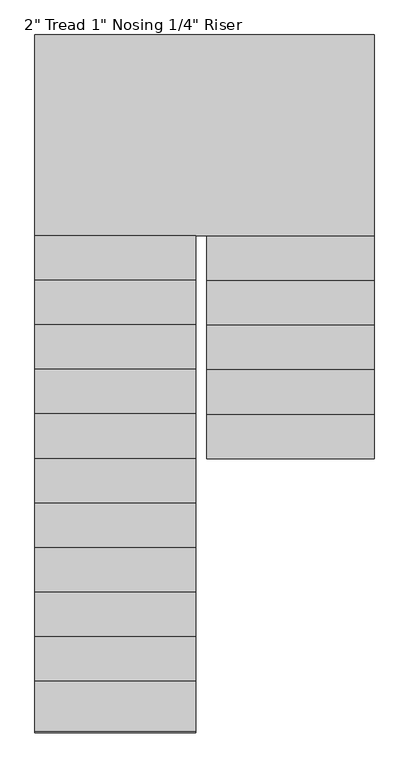
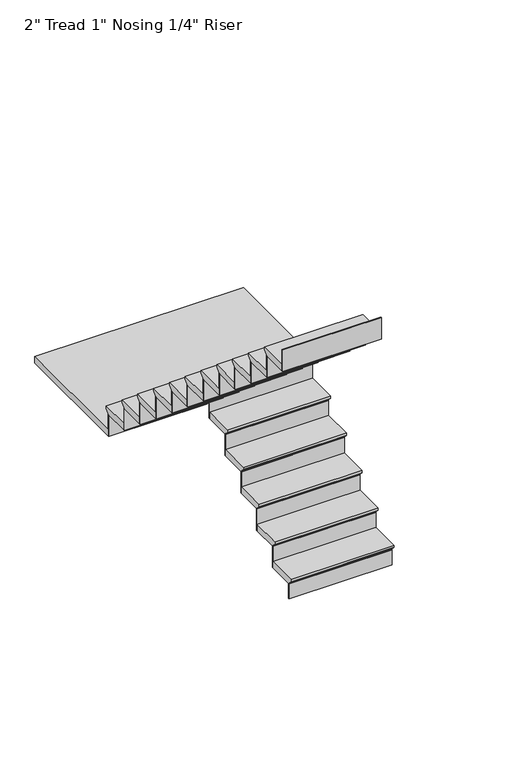
"""IFC4 building model written with IfcOpenShell, lengths in millimetres: stair flight geometry."""

from ifc_helpers import new_model, si_unit, origin, place, context, project, spatial, faceted_brep, source, transform, mapped, element, save


def stair_flight_cacad448(model_context):
    return source(origin(), model_context, "Body", "Brep", [
        faceted_brep([(-3749.597125, 2714.6319226, 27429.8833333), (-3749.597125, 2714.6319226, 27448.9333333), (-4512.2136682, 2714.6319226, 27448.9333333), (-4512.2136682, 2714.6319226, 27429.8833333), (-3749.597125, 2740.0319226, 27404.4833333), (-4512.2136682, 2740.0319226, 27404.4833333), (-3749.597125, 2943.2319226, 27448.9333333), (-4512.2136682, 2943.2319226, 27448.9333333), (-4512.2136682, 2740.0319226, 27398.1333333), (-4512.2136682, 2943.2319226, 27398.1333333), (-3749.597125, 2943.2319226, 27398.1333333), (-3749.597125, 2740.0319226, 27398.1333333)], [[[0, 1, 2, 3]], [[4, 0, 3, 5]], [[2, 1, 6, 7]], [[8, 9, 10, 11]], [[2, 7, 9, 8, 5, 3]], [[8, 11, 4, 5]], [[6, 1, 0, 4, 11, 10]], [[7, 6, 10, 9]]]),
        faceted_brep([(-3749.597125, 2740.0319226, 27398.1333333), (-3749.597125, 2740.0319226, 27279.6), (-3749.597125, 2746.3819226, 27279.6), (-3749.597125, 2746.3819226, 27398.1333333), (-4512.2136682, 2740.0319226, 27398.1333333), (-4512.2136682, 2746.3819226, 27398.1333333), (-4512.2136682, 2746.3819226, 27279.6), (-4512.2136682, 2740.0319226, 27279.6)], [[[0, 1, 2, 3]], [[4, 5, 6, 7]], [[1, 0, 4, 7]], [[2, 1, 7, 6]], [[3, 2, 6, 5]], [[0, 3, 5, 4]]]),
        faceted_brep([(-3749.597125, 2943.2319226, 27567.4666667), (-3749.597125, 2943.2319226, 27398.1333333), (-3749.597125, 2949.5819226, 27398.1333333), (-3749.597125, 2949.5819226, 27567.4666667), (-4512.2136682, 2943.2319226, 27567.4666667), (-4512.2136682, 2949.5819226, 27567.4666667), (-4512.2136682, 2949.5819226, 27398.1333333), (-4512.2136682, 2943.2319226, 27398.1333333)], [[[0, 1, 2, 3]], [[4, 5, 6, 7]], [[1, 0, 4, 7]], [[2, 1, 7, 6]], [[3, 2, 6, 5]], [[0, 3, 5, 4]]]),
        faceted_brep([(-4512.2136682, 2917.8319226, 27618.2666667), (-3749.597125, 2917.8319226, 27618.2666667), (-3749.597125, 3146.4319226, 27618.2666667), (-4512.2136682, 3146.4319226, 27618.2666667), (-4512.2136682, 2943.2319226, 27567.4666667), (-4512.2136682, 3146.4319226, 27567.4666667), (-3749.597125, 3146.4319226, 27567.4666667), (-3749.597125, 2943.2319226, 27567.4666667), (-4512.2136682, 2943.2319226, 27573.8166667), (-4512.2136682, 2917.8319226, 27599.2166667), (-3749.597125, 2943.2319226, 27573.8166667), (-3749.597125, 2917.8319226, 27599.2166667)], [[[0, 1, 2, 3]], [[4, 5, 6, 7]], [[0, 3, 5, 4, 8, 9]], [[4, 7, 10, 8]], [[2, 1, 11, 10, 7, 6]], [[3, 2, 6, 5]], [[11, 1, 0, 9]], [[10, 11, 9, 8]]]),
        faceted_brep([(-3749.597125, 3146.4319226, 27736.8), (-3749.597125, 3146.4319226, 27567.4666667), (-3749.597125, 3152.7819226, 27567.4666667), (-3749.597125, 3152.7819226, 27736.8), (-4512.2136682, 3146.4319226, 27736.8), (-4512.2136682, 3152.7819226, 27736.8), (-4512.2136682, 3152.7819226, 27567.4666667), (-4512.2136682, 3146.4319226, 27567.4666667)], [[[0, 1, 2, 3]], [[4, 5, 6, 7]], [[1, 0, 4, 7]], [[2, 1, 7, 6]], [[3, 2, 6, 5]], [[0, 3, 5, 4]]]),
        faceted_brep([(-4512.2136682, 3121.0319226, 27787.6), (-3749.597125, 3121.0319226, 27787.6), (-3749.597125, 3349.6319226, 27787.6), (-4512.2136682, 3349.6319226, 27787.6), (-4512.2136682, 3146.4319226, 27736.8), (-4512.2136682, 3349.6319226, 27736.8), (-3749.597125, 3349.6319226, 27736.8), (-3749.597125, 3146.4319226, 27736.8), (-4512.2136682, 3146.4319226, 27743.15), (-4512.2136682, 3121.0319226, 27768.55), (-3749.597125, 3146.4319226, 27743.15), (-3749.597125, 3121.0319226, 27768.55)], [[[0, 1, 2, 3]], [[4, 5, 6, 7]], [[0, 3, 5, 4, 8, 9]], [[4, 7, 10, 8]], [[2, 1, 11, 10, 7, 6]], [[3, 2, 6, 5]], [[11, 1, 0, 9]], [[10, 11, 9, 8]]]),
        faceted_brep([(-3749.597125, 3349.6319226, 27906.1333333), (-3749.597125, 3349.6319226, 27736.8), (-3749.597125, 3355.9819226, 27736.8), (-3749.597125, 3355.9819226, 27906.1333333), (-4512.2136682, 3349.6319226, 27906.1333333), (-4512.2136682, 3355.9819226, 27906.1333333), (-4512.2136682, 3355.9819226, 27736.8), (-4512.2136682, 3349.6319226, 27736.8)], [[[0, 1, 2, 3]], [[4, 5, 6, 7]], [[1, 0, 4, 7]], [[2, 1, 7, 6]], [[3, 2, 6, 5]], [[0, 3, 5, 4]]]),
        faceted_brep([(-4512.2136682, 3324.2319226, 27956.9333333), (-3749.597125, 3324.2319226, 27956.9333333), (-3749.597125, 3552.8319226, 27956.9333333), (-4512.2136682, 3552.8319226, 27956.9333333), (-4512.2136682, 3349.6319226, 27906.1333333), (-4512.2136682, 3552.8319226, 27906.1333333), (-3749.597125, 3552.8319226, 27906.1333333), (-3749.597125, 3349.6319226, 27906.1333333), (-4512.2136682, 3349.6319226, 27912.4833333), (-4512.2136682, 3324.2319226, 27937.8833333), (-3749.597125, 3349.6319226, 27912.4833333), (-3749.597125, 3324.2319226, 27937.8833333)], [[[0, 1, 2, 3]], [[4, 5, 6, 7]], [[0, 3, 5, 4, 8, 9]], [[4, 7, 10, 8]], [[2, 1, 11, 10, 7, 6]], [[3, 2, 6, 5]], [[11, 1, 0, 9]], [[10, 11, 9, 8]]]),
        faceted_brep([(-3749.597125, 3552.8319226, 28075.4666667), (-3749.597125, 3552.8319226, 27906.1333333), (-3749.597125, 3559.1819226, 27906.1333333), (-3749.597125, 3559.1819226, 28075.4666667), (-4512.2136682, 3552.8319226, 28075.4666667), (-4512.2136682, 3559.1819226, 28075.4666667), (-4512.2136682, 3559.1819226, 27906.1333333), (-4512.2136682, 3552.8319226, 27906.1333333)], [[[0, 1, 2, 3]], [[4, 5, 6, 7]], [[1, 0, 4, 7]], [[2, 1, 7, 6]], [[3, 2, 6, 5]], [[0, 3, 5, 4]]]),
        faceted_brep([(-4512.2136682, 3527.4319226, 28126.2666667), (-3749.597125, 3527.4319226, 28126.2666667), (-3749.597125, 3756.0319226, 28126.2666667), (-4512.2136682, 3756.0319226, 28126.2666667), (-4512.2136682, 3552.8319226, 28075.4666667), (-4512.2136682, 3756.0319226, 28075.4666667), (-3749.597125, 3756.0319226, 28075.4666667), (-3749.597125, 3552.8319226, 28075.4666667), (-4512.2136682, 3552.8319226, 28081.8166667), (-4512.2136682, 3527.4319226, 28107.2166667), (-3749.597125, 3552.8319226, 28081.8166667), (-3749.597125, 3527.4319226, 28107.2166667)], [[[0, 1, 2, 3]], [[4, 5, 6, 7]], [[0, 3, 5, 4, 8, 9]], [[4, 7, 10, 8]], [[2, 1, 11, 10, 7, 6]], [[3, 2, 6, 5]], [[11, 1, 0, 9]], [[10, 11, 9, 8]]]),
        faceted_brep([(-3749.597125, 3756.0319226, 28244.8), (-3749.597125, 3756.0319226, 28075.4666667), (-3749.597125, 3762.3819226, 28075.4666667), (-3749.597125, 3762.3819226, 28244.8), (-4512.2136682, 3756.0319226, 28244.8), (-4512.2136682, 3762.3819226, 28244.8), (-4512.2136682, 3762.3819226, 28075.4666667), (-4512.2136682, 3756.0319226, 28075.4666667)], [[[0, 1, 2, 3]], [[4, 5, 6, 7]], [[1, 0, 4, 7]], [[2, 1, 7, 6]], [[3, 2, 6, 5]], [[0, 3, 5, 4]]]),
        faceted_brep([(-4563.0136682, 3705.2319226, 28295.6), (-4563.0136682, 3730.6319226, 28295.6), (-3749.597125, 3730.6319226, 28295.6), (-3749.597125, 4645.0319226, 28295.6), (-5295.0246464, 4645.0319226, 28295.6), (-5295.0246464, 3705.2319226, 28295.6), (-4563.0136682, 3730.6319226, 28244.8), (-4563.0136682, 3705.2319226, 28244.8), (-5295.0246464, 3705.2319226, 28244.8), (-5295.0246464, 4645.0319226, 28244.8), (-3749.597125, 4645.0319226, 28244.8), (-3749.597125, 3756.0319226, 28244.8), (-4512.2136682, 3756.0319226, 28244.8), (-4512.2136682, 3730.6319226, 28244.8), (-4512.2136682, 3730.6319226, 28276.55), (-3749.597125, 3730.6319226, 28276.55), (-4512.2136682, 3756.0319226, 28251.15), (-3749.597125, 3756.0319226, 28251.15)], [[[0, 1, 2, 3, 4, 5]], [[6, 7, 8, 9, 10, 11, 12, 13]], [[1, 0, 7, 6]], [[2, 1, 6, 13, 14, 15]], [[13, 12, 16, 14]], [[12, 11, 17, 16]], [[3, 2, 15, 17, 11, 10]], [[4, 3, 10, 9]], [[5, 4, 9, 8]], [[0, 5, 8, 7]], [[17, 15, 14, 16]]]),
        faceted_brep([(-5295.0246464, 3705.2319226, 28414.1333333), (-5295.0246464, 3705.2319226, 28244.8), (-5295.0246464, 3698.8819226, 28244.8), (-5295.0246464, 3698.8819226, 28414.1333333), (-4563.0136682, 3705.2319226, 28414.1333333), (-4563.0136682, 3698.8819226, 28414.1333333), (-4563.0136682, 3698.8819226, 28244.8), (-4563.0136682, 3705.2319226, 28244.8)], [[[0, 1, 2, 3]], [[4, 5, 6, 7]], [[1, 0, 4, 7]], [[2, 1, 7, 6]], [[3, 2, 6, 5]], [[0, 3, 5, 4]]]),
        faceted_brep([(-4563.0136682, 3730.6319226, 28464.9333333), (-5295.0246464, 3730.6319226, 28464.9333333), (-5295.0246464, 3502.0319226, 28464.9333333), (-4563.0136682, 3502.0319226, 28464.9333333), (-4563.0136682, 3705.2319226, 28414.1333333), (-4563.0136682, 3502.0319226, 28414.1333333), (-5295.0246464, 3502.0319226, 28414.1333333), (-5295.0246464, 3705.2319226, 28414.1333333), (-4563.0136682, 3705.2319226, 28420.4833333), (-4563.0136682, 3730.6319226, 28445.8833333), (-5295.0246464, 3705.2319226, 28420.4833333), (-5295.0246464, 3730.6319226, 28445.8833333)], [[[0, 1, 2, 3]], [[4, 5, 6, 7]], [[0, 3, 5, 4, 8, 9]], [[4, 7, 10, 8]], [[2, 1, 11, 10, 7, 6]], [[3, 2, 6, 5]], [[11, 1, 0, 9]], [[10, 11, 9, 8]]]),
        faceted_brep([(-5295.0246464, 3502.0319226, 28583.4666667), (-5295.0246464, 3502.0319226, 28414.1333333), (-5295.0246464, 3495.6819226, 28414.1333333), (-5295.0246464, 3495.6819226, 28583.4666667), (-4563.0136682, 3502.0319226, 28583.4666667), (-4563.0136682, 3495.6819226, 28583.4666667), (-4563.0136682, 3495.6819226, 28414.1333333), (-4563.0136682, 3502.0319226, 28414.1333333)], [[[0, 1, 2, 3]], [[4, 5, 6, 7]], [[1, 0, 4, 7]], [[2, 1, 7, 6]], [[3, 2, 6, 5]], [[0, 3, 5, 4]]]),
        faceted_brep([(-4563.0136682, 3527.4319226, 28634.2666667), (-5295.0246464, 3527.4319226, 28634.2666667), (-5295.0246464, 3298.8319226, 28634.2666667), (-4563.0136682, 3298.8319226, 28634.2666667), (-4563.0136682, 3502.0319226, 28583.4666667), (-4563.0136682, 3298.8319226, 28583.4666667), (-5295.0246464, 3298.8319226, 28583.4666667), (-5295.0246464, 3502.0319226, 28583.4666667), (-4563.0136682, 3502.0319226, 28589.8166667), (-4563.0136682, 3527.4319226, 28615.2166667), (-5295.0246464, 3502.0319226, 28589.8166667), (-5295.0246464, 3527.4319226, 28615.2166667)], [[[0, 1, 2, 3]], [[4, 5, 6, 7]], [[0, 3, 5, 4, 8, 9]], [[4, 7, 10, 8]], [[2, 1, 11, 10, 7, 6]], [[3, 2, 6, 5]], [[11, 1, 0, 9]], [[10, 11, 9, 8]]]),
        faceted_brep([(-5295.0246464, 3298.8319226, 28752.8), (-5295.0246464, 3298.8319226, 28583.4666667), (-5295.0246464, 3292.4819226, 28583.4666667), (-5295.0246464, 3292.4819226, 28752.8), (-4563.0136682, 3298.8319226, 28752.8), (-4563.0136682, 3292.4819226, 28752.8), (-4563.0136682, 3292.4819226, 28583.4666667), (-4563.0136682, 3298.8319226, 28583.4666667)], [[[0, 1, 2, 3]], [[4, 5, 6, 7]], [[1, 0, 4, 7]], [[2, 1, 7, 6]], [[3, 2, 6, 5]], [[0, 3, 5, 4]]]),
        faceted_brep([(-4563.0136682, 3324.2319226, 28803.6), (-5295.0246464, 3324.2319226, 28803.6), (-5295.0246464, 3095.6319226, 28803.6), (-4563.0136682, 3095.6319226, 28803.6), (-4563.0136682, 3298.8319226, 28752.8), (-4563.0136682, 3095.6319226, 28752.8), (-5295.0246464, 3095.6319226, 28752.8), (-5295.0246464, 3298.8319226, 28752.8), (-4563.0136682, 3298.8319226, 28759.15), (-4563.0136682, 3324.2319226, 28784.55), (-5295.0246464, 3298.8319226, 28759.15), (-5295.0246464, 3324.2319226, 28784.55)], [[[0, 1, 2, 3]], [[4, 5, 6, 7]], [[0, 3, 5, 4, 8, 9]], [[4, 7, 10, 8]], [[2, 1, 11, 10, 7, 6]], [[3, 2, 6, 5]], [[11, 1, 0, 9]], [[10, 11, 9, 8]]]),
        faceted_brep([(-5295.0246464, 3095.6319226, 28922.1333333), (-5295.0246464, 3095.6319226, 28752.8), (-5295.0246464, 3089.2819226, 28752.8), (-5295.0246464, 3089.2819226, 28922.1333333), (-4563.0136682, 3095.6319226, 28922.1333333), (-4563.0136682, 3089.2819226, 28922.1333333), (-4563.0136682, 3089.2819226, 28752.8), (-4563.0136682, 3095.6319226, 28752.8)], [[[0, 1, 2, 3]], [[4, 5, 6, 7]], [[1, 0, 4, 7]], [[2, 1, 7, 6]], [[3, 2, 6, 5]], [[0, 3, 5, 4]]]),
        faceted_brep([(-4563.0136682, 3121.0319226, 28972.9333333), (-5295.0246464, 3121.0319226, 28972.9333333), (-5295.0246464, 2892.4319226, 28972.9333333), (-4563.0136682, 2892.4319226, 28972.9333333), (-4563.0136682, 3095.6319226, 28922.1333333), (-4563.0136682, 2892.4319226, 28922.1333333), (-5295.0246464, 2892.4319226, 28922.1333333), (-5295.0246464, 3095.6319226, 28922.1333333), (-4563.0136682, 3095.6319226, 28928.4833333), (-4563.0136682, 3121.0319226, 28953.8833333), (-5295.0246464, 3095.6319226, 28928.4833333), (-5295.0246464, 3121.0319226, 28953.8833333)], [[[0, 1, 2, 3]], [[4, 5, 6, 7]], [[0, 3, 5, 4, 8, 9]], [[4, 7, 10, 8]], [[2, 1, 11, 10, 7, 6]], [[3, 2, 6, 5]], [[11, 1, 0, 9]], [[10, 11, 9, 8]]]),
        faceted_brep([(-5295.0246464, 2892.4319226, 29091.4666667), (-5295.0246464, 2892.4319226, 28922.1333333), (-5295.0246464, 2886.0819226, 28922.1333333), (-5295.0246464, 2886.0819226, 29091.4666667), (-4563.0136682, 2892.4319226, 29091.4666667), (-4563.0136682, 2886.0819226, 29091.4666667), (-4563.0136682, 2886.0819226, 28922.1333333), (-4563.0136682, 2892.4319226, 28922.1333333)], [[[0, 1, 2, 3]], [[4, 5, 6, 7]], [[1, 0, 4, 7]], [[2, 1, 7, 6]], [[3, 2, 6, 5]], [[0, 3, 5, 4]]]),
        faceted_brep([(-4563.0136682, 2917.8319226, 29142.2666667), (-5295.0246464, 2917.8319226, 29142.2666667), (-5295.0246464, 2689.2319226, 29142.2666667), (-4563.0136682, 2689.2319226, 29142.2666667), (-4563.0136682, 2892.4319226, 29091.4666667), (-4563.0136682, 2689.2319226, 29091.4666667), (-5295.0246464, 2689.2319226, 29091.4666667), (-5295.0246464, 2892.4319226, 29091.4666667), (-4563.0136682, 2892.4319226, 29097.8166667), (-4563.0136682, 2917.8319226, 29123.2166667), (-5295.0246464, 2892.4319226, 29097.8166667), (-5295.0246464, 2917.8319226, 29123.2166667)], [[[0, 1, 2, 3]], [[4, 5, 6, 7]], [[0, 3, 5, 4, 8, 9]], [[4, 7, 10, 8]], [[2, 1, 11, 10, 7, 6]], [[3, 2, 6, 5]], [[11, 1, 0, 9]], [[10, 11, 9, 8]]]),
        faceted_brep([(-5295.0246464, 2689.2319226, 29260.8), (-5295.0246464, 2689.2319226, 29091.4666667), (-5295.0246464, 2682.8819226, 29091.4666667), (-5295.0246464, 2682.8819226, 29260.8), (-4563.0136682, 2689.2319226, 29260.8), (-4563.0136682, 2682.8819226, 29260.8), (-4563.0136682, 2682.8819226, 29091.4666667), (-4563.0136682, 2689.2319226, 29091.4666667)], [[[0, 1, 2, 3]], [[4, 5, 6, 7]], [[1, 0, 4, 7]], [[2, 1, 7, 6]], [[3, 2, 6, 5]], [[0, 3, 5, 4]]]),
        faceted_brep([(-4563.0136682, 2714.6319226, 29311.6), (-5295.0246464, 2714.6319226, 29311.6), (-5295.0246464, 2486.0319226, 29311.6), (-4563.0136682, 2486.0319226, 29311.6), (-4563.0136682, 2689.2319226, 29260.8), (-4563.0136682, 2486.0319226, 29260.8), (-5295.0246464, 2486.0319226, 29260.8), (-5295.0246464, 2689.2319226, 29260.8), (-4563.0136682, 2689.2319226, 29267.15), (-4563.0136682, 2714.6319226, 29292.55), (-5295.0246464, 2689.2319226, 29267.15), (-5295.0246464, 2714.6319226, 29292.55)], [[[0, 1, 2, 3]], [[4, 5, 6, 7]], [[0, 3, 5, 4, 8, 9]], [[4, 7, 10, 8]], [[2, 1, 11, 10, 7, 6]], [[3, 2, 6, 5]], [[11, 1, 0, 9]], [[10, 11, 9, 8]]]),
        faceted_brep([(-5295.0246464, 2486.0319226, 29430.1333333), (-5295.0246464, 2486.0319226, 29260.8), (-5295.0246464, 2479.6819226, 29260.8), (-5295.0246464, 2479.6819226, 29430.1333333), (-4563.0136682, 2486.0319226, 29430.1333333), (-4563.0136682, 2479.6819226, 29430.1333333), (-4563.0136682, 2479.6819226, 29260.8), (-4563.0136682, 2486.0319226, 29260.8)], [[[0, 1, 2, 3]], [[4, 5, 6, 7]], [[1, 0, 4, 7]], [[2, 1, 7, 6]], [[3, 2, 6, 5]], [[0, 3, 5, 4]]]),
        faceted_brep([(-4563.0136682, 2511.4319226, 29480.9333333), (-5295.0246464, 2511.4319226, 29480.9333333), (-5295.0246464, 2282.8319226, 29480.9333333), (-4563.0136682, 2282.8319226, 29480.9333333), (-4563.0136682, 2486.0319226, 29430.1333333), (-4563.0136682, 2282.8319226, 29430.1333333), (-5295.0246464, 2282.8319226, 29430.1333333), (-5295.0246464, 2486.0319226, 29430.1333333), (-4563.0136682, 2486.0319226, 29436.4833333), (-4563.0136682, 2511.4319226, 29461.8833333), (-5295.0246464, 2486.0319226, 29436.4833333), (-5295.0246464, 2511.4319226, 29461.8833333)], [[[0, 1, 2, 3]], [[4, 5, 6, 7]], [[0, 3, 5, 4, 8, 9]], [[4, 7, 10, 8]], [[2, 1, 11, 10, 7, 6]], [[3, 2, 6, 5]], [[11, 1, 0, 9]], [[10, 11, 9, 8]]]),
        faceted_brep([(-5295.0246464, 2282.8319226, 29599.4666667), (-5295.0246464, 2282.8319226, 29430.1333333), (-5295.0246464, 2276.4819226, 29430.1333333), (-5295.0246464, 2276.4819226, 29599.4666667), (-4563.0136682, 2282.8319226, 29599.4666667), (-4563.0136682, 2276.4819226, 29599.4666667), (-4563.0136682, 2276.4819226, 29430.1333333), (-4563.0136682, 2282.8319226, 29430.1333333)], [[[0, 1, 2, 3]], [[4, 5, 6, 7]], [[1, 0, 4, 7]], [[2, 1, 7, 6]], [[3, 2, 6, 5]], [[0, 3, 5, 4]]]),
        faceted_brep([(-4563.0136682, 2308.2319226, 29650.2666667), (-5295.0246464, 2308.2319226, 29650.2666667), (-5295.0246464, 2079.6319226, 29650.2666667), (-4563.0136682, 2079.6319226, 29650.2666667), (-4563.0136682, 2282.8319226, 29599.4666667), (-4563.0136682, 2079.6319226, 29599.4666667), (-5295.0246464, 2079.6319226, 29599.4666667), (-5295.0246464, 2282.8319226, 29599.4666667), (-4563.0136682, 2282.8319226, 29605.8166667), (-4563.0136682, 2308.2319226, 29631.2166667), (-5295.0246464, 2282.8319226, 29605.8166667), (-5295.0246464, 2308.2319226, 29631.2166667)], [[[0, 1, 2, 3]], [[4, 5, 6, 7]], [[0, 3, 5, 4, 8, 9]], [[4, 7, 10, 8]], [[2, 1, 11, 10, 7, 6]], [[3, 2, 6, 5]], [[11, 1, 0, 9]], [[10, 11, 9, 8]]]),
        faceted_brep([(-5295.0246464, 2079.6319226, 29768.8), (-5295.0246464, 2079.6319226, 29599.4666667), (-5295.0246464, 2073.2819226, 29599.4666667), (-5295.0246464, 2073.2819226, 29768.8), (-4563.0136682, 2079.6319226, 29768.8), (-4563.0136682, 2073.2819226, 29768.8), (-4563.0136682, 2073.2819226, 29599.4666667), (-4563.0136682, 2079.6319226, 29599.4666667)], [[[0, 1, 2, 3]], [[4, 5, 6, 7]], [[1, 0, 4, 7]], [[2, 1, 7, 6]], [[3, 2, 6, 5]], [[0, 3, 5, 4]]]),
        faceted_brep([(-4563.0136682, 2105.0319226, 29819.6), (-5295.0246464, 2105.0319226, 29819.6), (-5295.0246464, 1876.4319226, 29819.6), (-4563.0136682, 1876.4319226, 29819.6), (-4563.0136682, 2079.6319226, 29768.8), (-4563.0136682, 1876.4319226, 29768.8), (-5295.0246464, 1876.4319226, 29768.8), (-5295.0246464, 2079.6319226, 29768.8), (-4563.0136682, 2079.6319226, 29775.15), (-4563.0136682, 2105.0319226, 29800.55), (-5295.0246464, 2079.6319226, 29775.15), (-5295.0246464, 2105.0319226, 29800.55)], [[[0, 1, 2, 3]], [[4, 5, 6, 7]], [[0, 3, 5, 4, 8, 9]], [[4, 7, 10, 8]], [[2, 1, 11, 10, 7, 6]], [[3, 2, 6, 5]], [[11, 1, 0, 9]], [[10, 11, 9, 8]]]),
        faceted_brep([(-5295.0246464, 1876.4319226, 29938.1333333), (-5295.0246464, 1876.4319226, 29768.8), (-5295.0246464, 1870.0819226, 29768.8), (-5295.0246464, 1870.0819226, 29938.1333333), (-4563.0136682, 1876.4319226, 29938.1333333), (-4563.0136682, 1870.0819226, 29938.1333333), (-4563.0136682, 1870.0819226, 29768.8), (-4563.0136682, 1876.4319226, 29768.8)], [[[0, 1, 2, 3]], [[4, 5, 6, 7]], [[1, 0, 4, 7]], [[2, 1, 7, 6]], [[3, 2, 6, 5]], [[0, 3, 5, 4]]]),
        faceted_brep([(-4563.0136682, 1901.8319226, 29988.9333333), (-5295.0246464, 1901.8319226, 29988.9333333), (-5295.0246464, 1673.2319226, 29988.9333333), (-4563.0136682, 1673.2319226, 29988.9333333), (-4563.0136682, 1876.4319226, 29938.1333333), (-4563.0136682, 1673.2319226, 29938.1333333), (-5295.0246464, 1673.2319226, 29938.1333333), (-5295.0246464, 1876.4319226, 29938.1333333), (-4563.0136682, 1876.4319226, 29944.4833333), (-4563.0136682, 1901.8319226, 29969.8833333), (-5295.0246464, 1876.4319226, 29944.4833333), (-5295.0246464, 1901.8319226, 29969.8833333)], [[[0, 1, 2, 3]], [[4, 5, 6, 7]], [[0, 3, 5, 4, 8, 9]], [[4, 7, 10, 8]], [[2, 1, 11, 10, 7, 6]], [[3, 2, 6, 5]], [[11, 1, 0, 9]], [[10, 11, 9, 8]]]),
        faceted_brep([(-5295.0246464, 1673.2319226, 30107.4666667), (-5295.0246464, 1673.2319226, 29938.1333333), (-5295.0246464, 1666.8819226, 29938.1333333), (-5295.0246464, 1666.8819226, 30107.4666667), (-4563.0136682, 1673.2319226, 30107.4666667), (-4563.0136682, 1666.8819226, 30107.4666667), (-4563.0136682, 1666.8819226, 29938.1333333), (-4563.0136682, 1673.2319226, 29938.1333333)], [[[0, 1, 2, 3]], [[4, 5, 6, 7]], [[1, 0, 4, 7]], [[2, 1, 7, 6]], [[3, 2, 6, 5]], [[0, 3, 5, 4]]]),
        faceted_brep([(-4563.0136682, 1698.6319226, 30158.2666667), (-5295.0246464, 1698.6319226, 30158.2666667), (-5295.0246464, 1470.0319226, 30158.2666667), (-4563.0136682, 1470.0319226, 30158.2666667), (-4563.0136682, 1673.2319226, 30107.4666667), (-4563.0136682, 1470.0319226, 30107.4666667), (-5295.0246464, 1470.0319226, 30107.4666667), (-5295.0246464, 1673.2319226, 30107.4666667), (-4563.0136682, 1673.2319226, 30113.8166667), (-4563.0136682, 1698.6319226, 30139.2166667), (-5295.0246464, 1673.2319226, 30113.8166667), (-5295.0246464, 1698.6319226, 30139.2166667)], [[[0, 1, 2, 3]], [[4, 5, 6, 7]], [[0, 3, 5, 4, 8, 9]], [[4, 7, 10, 8]], [[2, 1, 11, 10, 7, 6]], [[3, 2, 6, 5]], [[11, 1, 0, 9]], [[10, 11, 9, 8]]]),
        faceted_brep([(-5295.0246464, 1470.0319226, 30276.8), (-5295.0246464, 1470.0319226, 30107.4666667), (-5295.0246464, 1463.6819226, 30107.4666667), (-5295.0246464, 1463.6819226, 30276.8), (-4563.0136682, 1470.0319226, 30276.8), (-4563.0136682, 1463.6819226, 30276.8), (-4563.0136682, 1463.6819226, 30107.4666667), (-4563.0136682, 1470.0319226, 30107.4666667)], [[[0, 1, 2, 3]], [[4, 5, 6, 7]], [[1, 0, 4, 7]], [[2, 1, 7, 6]], [[3, 2, 6, 5]], [[0, 3, 5, 4]]]),
    ])


if __name__ == "__main__":
    model = new_model("IFC4")
    model_context = context("Model", 3, world=origin())
    ifc_project = project(units=[si_unit("LENGTHUNIT", "METRE", prefix="MILLI")], contexts=[model_context])
    site = spatial("IfcSite", under=ifc_project)
    building = spatial("IfcBuilding", under=site)
    placement = place(None, origin())
    stair_flight_shape = stair_flight_cacad448(model_context)
    element("IfcStairFlight", 1, ObjectType="2\" Tread 1\" Nosing 1/4\" Riser", at=placement, inside=building, context=model_context, shape_type="MappedRepresentation", body=[
        mapped(stair_flight_shape, transform((0.0, 0.0, 0.0), x_axis=(1.0, 0.0, 0.0), y_axis=(0.0, 1.0, 0.0), z_axis=(0.0, 0.0, 1.0))),
    ])
    save(model, "model.ifc")
